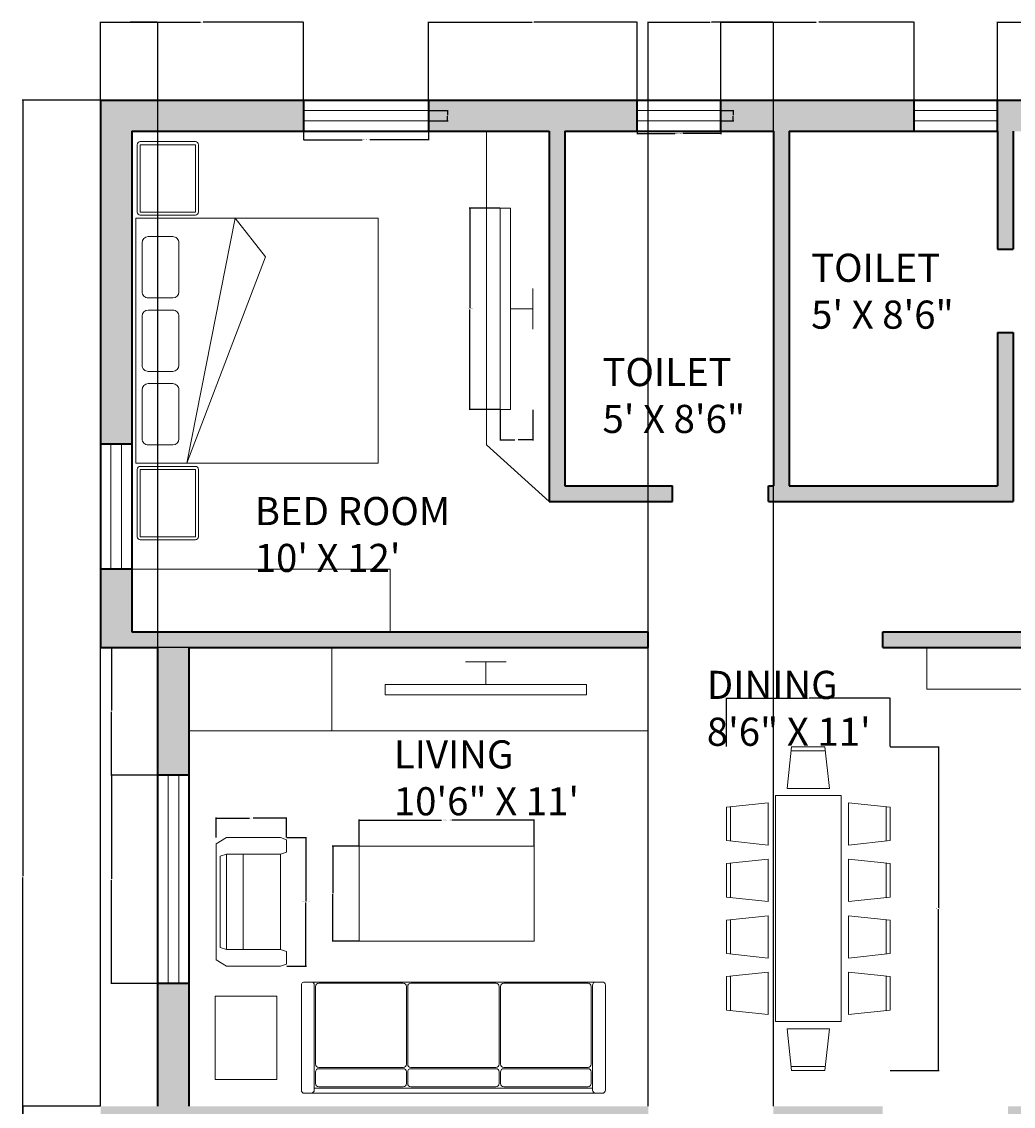
# Model space of a CAD drawing. Units: inches. Extents: x 2 to 2806, y 1095 to 1587.
# Tile 3 of 4: x 2363 to 2648, y 1275 to 1587. Entities that reach past the tile are written whole.
import ezdxf

# ---------------------------------------------------------------- set-up
doc = ezdxf.new("R2010")
doc.units = ezdxf.units.IN
for name, color, linetype, lineweight in [('A-ANNO-DIMS', 2, 'Continuous', 18), ('A-AREA-IDEN', 7, 'Continuous', 25), ('A-EQPM', 8, 'Continuous', 18), ('A-FLOR-CASE', 34, 'Continuous', 18), ('A-FURN', 8, 'Continuous', 18), ('A-GLAZ', 4, 'Continuous', 18), ('A-WALL', 7, 'Continuous', 35)]:
    doc.layers.add(name, color=color, linetype=linetype, lineweight=lineweight)
doc.layers.add('A-WALL-PATT', color=18, linetype='Continuous', lineweight=13, true_color=0x000000)
doc.styles.get("Standard").update_dxf_attribs({"font": 'arial.ttf'})
doc.dimstyles.get("Standard").update_dxf_attribs({"dimtxt": 0.18, "dimasz": 0.18, "dimexe": 0.18, "dimexo": 0.0625, "dimgap": 0.09, "dimtad": 0, "dimtih": 1, "dimtoh": 1, "dimdec": 4, "dimzin": 0, "dimdsep": 46, "dimtxsty": 'Standard', "dimcen": 0.09, "dimadec": 0, "dimazin": 0, "dimtfac": 1, "dimtdec": 4, "dimtofl": 0, "dimtmove": 0, "dimatfit": 3, "dimfxl": 1, "dimtolj": 1, "dimtzin": 0, "dimarcsym": 0})

# ---------------------------------------------------------------- blocks, each defined once
blk = doc.blocks.new('A$C5E814E7E')
for p, q in [((0.593, 1.293), (0.64, 1.736)), ((0.64, 1.736), (0.995, 1.736)), ((0.995, 1.736), (1.043, 1.293)), ((1.193, 1.293), (1.24, 1.736)), ((1.24, 1.736), (1.595, 1.736)), ((1.595, 1.736), (1.643, 1.293)), ((1.793, 1.293), (1.84, 1.736)), ((1.84, 1.736), (2.195, 1.736)), ((2.195, 1.736), (2.243, 1.293)), ((2.393, 1.293), (2.44, 1.736)), ((2.44, 1.736), (2.795, 1.736)), ((2.795, 1.736), (2.843, 1.293)), ((0.636, 1.693), (1, 1.693)), ((1.236, 1.693), (1.6, 1.693)), ((1.836, 1.693), (2.2, 1.693)), ((2.436, 1.693), (2.8, 1.693)), ((1.043, 1.293), (0.593, 1.293)), ((1.643, 1.293), (1.193, 1.293)), ((2.243, 1.293), (1.793, 1.293)), ((2.843, 1.293), (2.393, 1.293)), ((0.518, 1.218), (2.918, 1.218)), ((0.518, 0.518), (0.518, 1.218)), ((2.918, 1.218), (2.918, 0.518)), ((0.443, 1.093), (0, 1.045)), ((0, 1.045), (0, 0.69)), ((0.043, 1.05), (0.043, 0.686)), ((0.443, 0.643), (0.443, 1.093)), ((2.993, 1.093), (3.436, 1.045)), ((2.993, 0.643), (2.993, 1.093)), ((3.393, 1.05), (3.393, 0.686)), ((3.436, 1.045), (3.436, 0.69)), ((0, 0.69), (0.443, 0.643)), ((3.436, 0.69), (2.993, 0.643)), ((2.918, 0.518), (0.518, 0.518)), ((0.593, 0.443), (0.64, 0)), ((1.043, 0.443), (0.593, 0.443)), ((0.995, 0), (1.043, 0.443)), ((1.193, 0.443), (1.24, 0)), ((1.643, 0.443), (1.193, 0.443)), ((1.595, 0), (1.643, 0.443)), ((2.243, 0.443), (1.793, 0.443)), ((1.793, 0.443), (1.84, 0)), ((2.195, 0), (2.243, 0.443)), ((2.393, 0.443), (2.44, 0)), ((2.843, 0.443), (2.393, 0.443)), ((2.795, 0), (2.843, 0.443)), ((0.636, 0.043), (1, 0.043)), ((1.236, 0.043), (1.6, 0.043)), ((1.836, 0.043), (2.2, 0.043)), ((2.436, 0.043), (2.8, 0.043)), ((0.64, 0), (0.995, 0)), ((1.24, 0), (1.595, 0)), ((1.84, 0), (2.195, 0)), ((2.44, 0), (2.795, 0))]:
    blk.add_line(p, q)
blk = doc.blocks.new('A$C0BA509B0')
for p, q in [((0.025, 0.86), (2.325, 0.86)), ((2.25, 0.8385), (2.25, 0.0224)), ((0, 0.025), (0, 0.835)), ((0.1, 0.0219), (0.1, 0.8375)), ((0.1, 0.82), (2.25, 0.82)), ((0.11, 0.695), (0.11, 0.785)), ((0.135, 0.81), (0.7866, 0.81)), ((0.8116, 0.785), (0.8116, 0.695)), ((0.8216, 0.785), (0.8216, 0.695)), ((0.8466, 0.81), (1.5033, 0.81)), ((1.5283, 0.785), (1.5283, 0.695)), ((1.5383, 0.785), (1.5383, 0.695)), ((1.5633, 0.81), (2.215, 0.81)), ((2.24, 0.785), (2.24, 0.695)), ((2.35, 0.835), (2.35, 0.025)), ((0.11, 0.035), (0.11, 0.635)), ((0.135, 0.67), (0.7866, 0.67)), ((0.135, 0.66), (0.7866, 0.66)), ((0.8116, 0.635), (0.8116, 0.035)), ((0.8216, 0.635), (0.8216, 0.035)), ((0.8466, 0.67), (1.5033, 0.67)), ((0.8466, 0.66), (1.5033, 0.66)), ((1.5283, 0.635), (1.5283, 0.035)), ((1.5383, 0.635), (1.5383, 0.035)), ((1.5633, 0.67), (2.215, 0.67)), ((1.5633, 0.66), (2.215, 0.66)), ((2.24, 0.635), (2.24, 0.035)), ((0.7866, 0.01), (0.135, 0.01)), ((1.5033, 0.01), (0.8466, 0.01)), ((2.215, 0.01), (1.5633, 0.01)), ((2.325, 0), (0.025, 0))]:
    blk.add_line(p, q)
for centre, start, end in [((0.025, 0.835), 90, 180), ((0.0751, 0.835), 0, 90), ((2.2752, 0.835), 90, 180), ((2.325, 0.835), 0, 90), ((0.135, 0.785), 90, 180), ((0.7866, 0.785), 0, 90), ((0.8466, 0.785), 90, 180), ((1.5033, 0.785), 0, 90), ((1.5633, 0.785), 90, 180), ((2.215, 0.785), 0, 90), ((0.135, 0.695), 180, 270), ((0.7866, 0.695), 270, 0), ((0.8466, 0.695), 180, 270), ((1.5033, 0.695), 270, 0), ((1.5633, 0.695), 180, 270), ((2.215, 0.695), 270, 0), ((0.135, 0.635), 90, 180), ((0.7866, 0.635), 0, 90), ((0.8466, 0.635), 90, 180), ((1.5033, 0.635), 0, 90), ((1.5633, 0.635), 90, 180), ((2.215, 0.635), 0, 90), ((0.025, 0.025), 180, 270), ((0.0751, 0.025), 270, 0), ((0.135, 0.035), 180, 270), ((0.7866, 0.035), 270, 0), ((0.8466, 0.035), 180, 270), ((1.5033, 0.035), 270, 0), ((1.5633, 0.035), 180, 270), ((2.215, 0.035), 270, 0), ((2.2749, 0.025), 180, 270), ((2.325, 0.025), 270, 0)]:
    blk.add_arc(centre, 0.025, start, end)
blk = doc.blocks.new('A$C61201922')
for p, q in [((0, 0.737), (0.076, 0.864)), ((0.076, 0.864), (1.499, 0.864)), ((0.203, 0.737), (0.229, 0.813)), ((0.229, 0.813), (1.346, 0.813)), ((1.346, 0.813), (1.372, 0.737)), ((1.499, 0.864), (1.575, 0.737)), ((0, 0.076), (0, 0.737)), ((0.203, 0.076), (0.203, 0.737)), ((1.372, 0.737), (0.203, 0.737)), ((1.372, 0.737), (1.372, 0.076)), ((1.575, 0.737), (1.575, 0.076)), ((1.372, 0.533), (0.203, 0.533)), ((0.025, 0), (0, 0.076)), ((0.178, 0), (0.025, 0)), ((0.203, 0.076), (0.178, 0)), ((1.372, 0.076), (0.203, 0.076)), ((1.397, 0), (1.372, 0.076)), ((1.549, 0), (1.397, 0)), ((1.575, 0.076), (1.549, 0))]:
    blk.add_line(p, q)
blk = doc.blocks.new('A$C793B20D3')
for p, q in [((0.625, 0), (0.625, 1.975)), ((2.625, 1.975), (0.625, 1.975)), ((2.625, 0), (2.625, 1.975)), ((2.675, 1.9655), (3.225, 1.9655)), ((0.575, 1.9405), (0.025, 1.9405)), ((0.025, 1.9405), (0.025, 1.4905)), ((0.575, 1.4905), (0.575, 1.9405)), ((0.775, 1.675), (0.775, 1.875)), ((0.825, 1.925), (1.225, 1.925)), ((1.275, 1.675), (1.275, 1.875)), ((1.375, 1.675), (1.375, 1.875)), ((1.425, 1.925), (1.825, 1.925)), ((1.875, 1.675), (1.875, 1.875)), ((1.975, 1.675), (1.975, 1.875)), ((2.025, 1.925), (2.425, 1.925)), ((2.475, 1.675), (2.475, 1.875)), ((2.65, 1.4905), (2.65, 1.9405)), ((3.25, 1.9405), (3.25, 1.4905)), ((0.825, 1.625), (1.225, 1.625)), ((1.425, 1.625), (1.825, 1.625)), ((2.025, 1.625), (2.425, 1.625)), ((0.6256, 1.5604), (2.3107, 0.9169)), ((0.6256, 1.5604), (2.625, 1.1646)), ((0.025, 1.4905), (0.575, 1.4905)), ((3.225, 1.4655), (2.675, 1.4655)), ((2.3107, 0.9169), (2.625, 1.1646)), ((2.625, 0), (0.625, 0))]:
    blk.add_line(p, q)
at = {"flags": 128}
blk.add_lwpolyline([(0, 1.9405), (0, 1.4905, 0.414214), (0.025, 1.4655), (0.575, 1.4655, 0.414214), (0.6, 1.4905), (0.6, 1.9405, 0.414214), (0.575, 1.9655), (0.025, 1.9655, 0.414214)], format="xyb", close=True, dxfattribs=at)
blk.add_lwpolyline([(3.225, 1.9405), (3.225, 1.4905), (2.675, 1.4905), (2.675, 1.9405)], close=True)
for centre, radius, start, end in [((2.675, 1.9405), 0.025, 90, 180), ((3.225, 1.9405), 0.025, 0, 90), ((0.825, 1.875), 0.05, 90, 180), ((1.225, 1.875), 0.05, 0, 90), ((1.425, 1.875), 0.05, 90, 180), ((1.825, 1.875), 0.05, 0, 90), ((2.025, 1.875), 0.05, 90, 180), ((2.425, 1.875), 0.05, 0, 90), ((0.825, 1.675), 0.05, 180, 270), ((1.225, 1.675), 0.05, 270, 0), ((1.425, 1.675), 0.05, 180, 270), ((1.825, 1.675), 0.05, 270, 0), ((2.025, 1.675), 0.05, 180, 270), ((2.425, 1.675), 0.05, 270, 0), ((2.675, 1.4905), 0.025, 180, 270), ((3.225, 1.4905), 0.025, 270, 0)]:
    blk.add_arc(centre, radius, start, end)
blk = doc.blocks.new('WIN-GLAZ-36x9')
for p, q in [((0, 3), (36, 3)), ((0, 0), (36, 0))]:
    blk.add_line(p, q)
blk = doc.blocks.new('WIN-GLAZ-24x9')
for p, q in [((0, 3), (24, 3)), ((0, 0), (24, 0))]:
    blk.add_line(p, q)
blk = doc.blocks.new('TV-FLAT-PANEL')
for p, q in [((23.15, 9.45), (34.81, 9.45)), ((28.98, 3), (28.98, 9.45)), ((0, 3), (57.96, 3)), ((0, 3), (0, 0)), ((0, 0), (57.96, 0)), ((57.96, 0), (57.96, 3))]:
    blk.add_line(p, q)
blk = doc.blocks.new('TABLE-COFFEE-RECT')
blk.add_lwpolyline([(0, 27.27), (50.38, 27.27), (50.38, 0), (0, 0), (0, 27.27)])
blk = doc.blocks.new('*D26')
at = {"layer": 'A-ANNO-DIMS', "color": 0, "lineweight": -2, "transparency": 16777216}
for p, q in [((2444, 1558.15), (2444, 1552.63)), ((2480, 1558.15), (2480, 1552.63)), ((2444.18, 1552.81), (2460.88, 1552.81)), ((2479.82, 1552.81), (2463.12, 1552.81))]:
    blk.add_line(p, q, dxfattribs=at)
at = {"layer": 'A-ANNO-DIMS', "color": 0, "transparency": 16777216}
for points in [[(2444.18, 1552.84), (2444.18, 1552.78), (2444, 1552.81)], [(2479.82, 1552.84), (2479.82, 1552.78), (2480, 1552.81)]]:
    blk.add_solid(points, dxfattribs=at)
at = {"layer": 'Defpoints', "color": 0, "transparency": 16777216}
for p in [(2444, 1558.21), (2480, 1558.21), (2480, 1552.81)]:
    blk.add_point(p, dxfattribs=at)
at = {"layer": 'A-ANNO-DIMS', "color": 0, "transparency": 16777216, "insert": (2462, 1552.81), "char_height": 0.18, "attachment_point": 5}
blk.add_mtext('\\A1;WINDOW 36 TYP.', dxfattribs=at)
blk = doc.blocks.new('*D27')
at = {"layer": 'A-ANNO-DIMS', "color": 0, "lineweight": -2, "transparency": 16777216}
for p, q in [((2480.06, 1561.21), (2485.58, 1561.21)), ((2485.4, 1561.03), (2485.4, 1559.9)), ((2480.06, 1558.21), (2485.58, 1558.21)), ((2485.4, 1558.39), (2485.4, 1559.53))]:
    blk.add_line(p, q, dxfattribs=at)
at = {"layer": 'A-ANNO-DIMS', "color": 0, "transparency": 16777216}
for points in [[(2485.37, 1561.03), (2485.43, 1561.03), (2485.4, 1561.21)], [(2485.37, 1558.39), (2485.43, 1558.39), (2485.4, 1558.21)]]:
    blk.add_solid(points, dxfattribs=at)
at = {"layer": 'Defpoints', "color": 0, "transparency": 16777216}
for p in [(2480, 1561.21), (2485.4, 1561.21), (2480, 1558.21)]:
    blk.add_point(p, dxfattribs=at)
at = {"layer": 'A-ANNO-DIMS', "color": 0, "transparency": 16777216, "insert": (2485.4, 1559.71), "char_height": 0.18, "attachment_point": 5}
blk.add_mtext('\\A1;3 TYP.', dxfattribs=at)
blk = doc.blocks.new('*D28')
at = {"layer": 'A-ANNO-DIMS', "color": 0, "lineweight": -2, "transparency": 16777216}
for p, q in [((2540, 1558.15), (2540, 1554.43)), ((2564, 1558.15), (2564, 1554.43)), ((2540.18, 1554.61), (2550.88, 1554.61)), ((2563.82, 1554.61), (2553.12, 1554.61))]:
    blk.add_line(p, q, dxfattribs=at)
at = {"layer": 'A-ANNO-DIMS', "color": 0, "transparency": 16777216}
for points in [[(2540.18, 1554.64), (2540.18, 1554.58), (2540, 1554.61)], [(2563.82, 1554.64), (2563.82, 1554.58), (2564, 1554.61)]]:
    blk.add_solid(points, dxfattribs=at)
at = {"layer": 'Defpoints', "color": 0, "transparency": 16777216}
for p in [(2540, 1558.21), (2564, 1558.21), (2564, 1554.61)]:
    blk.add_point(p, dxfattribs=at)
at = {"layer": 'A-ANNO-DIMS', "color": 0, "transparency": 16777216, "insert": (2552, 1554.61), "char_height": 0.18, "attachment_point": 5}
blk.add_mtext('\\A1;WINDOW 24 TYP.', dxfattribs=at)
blk = doc.blocks.new('*D29')
at = {"layer": 'A-ANNO-DIMS', "color": 0, "lineweight": -2, "transparency": 16777216}
for p, q in [((2564.06, 1561.21), (2567.78, 1561.21)), ((2567.6, 1561.03), (2567.6, 1559.9)), ((2564.06, 1558.21), (2567.78, 1558.21)), ((2567.6, 1558.39), (2567.6, 1559.53))]:
    blk.add_line(p, q, dxfattribs=at)
at = {"layer": 'A-ANNO-DIMS', "color": 0, "transparency": 16777216}
for points in [[(2567.57, 1561.03), (2567.63, 1561.03), (2567.6, 1561.21)], [(2567.57, 1558.39), (2567.63, 1558.39), (2567.6, 1558.21)]]:
    blk.add_solid(points, dxfattribs=at)
at = {"layer": 'Defpoints', "color": 0, "transparency": 16777216}
for p in [(2564, 1561.21), (2567.6, 1561.21), (2564, 1558.21)]:
    blk.add_point(p, dxfattribs=at)
at = {"layer": 'A-ANNO-DIMS', "color": 0, "transparency": 16777216, "insert": (2567.6, 1559.71), "char_height": 0.18, "attachment_point": 5}
blk.add_mtext('\\A1;3 TYP.', dxfattribs=at)
blk = doc.blocks.new('*D36')
at = {"layer": 'A-ANNO-DIMS', "color": 0, "lineweight": -2, "transparency": 16777216}
for p, q in [((2439.22, 1352.03), (2444.88, 1352.03)), ((2444.7, 1351.85), (2444.7, 1333.72)), ((2444.7, 1315.22), (2444.7, 1333.35)), ((2439.22, 1315.04), (2444.88, 1315.04))]:
    blk.add_line(p, q, dxfattribs=at)
at = {"layer": 'A-ANNO-DIMS', "color": 0, "transparency": 16777216}
for points in [[(2444.67, 1351.85), (2444.73, 1351.85), (2444.7, 1352.03)], [(2444.67, 1315.22), (2444.73, 1315.22), (2444.7, 1315.04)]]:
    blk.add_solid(points, dxfattribs=at)
at = {"layer": 'Defpoints', "color": 0, "transparency": 16777216}
for p in [(2439.15, 1352.03), (2444.7, 1352.03), (2439.15, 1315.04)]:
    blk.add_point(p, dxfattribs=at)
at = {"layer": 'A-ANNO-DIMS', "color": 0, "transparency": 16777216, "insert": (2444.7, 1333.54), "char_height": 0.18, "attachment_point": 5}
blk.add_mtext('\\A1;ARMCHAIR 37 TYP.', dxfattribs=at)
blk = doc.blocks.new('*D37')
at = {"layer": 'A-ANNO-DIMS', "color": 0, "lineweight": -2, "transparency": 16777216}
for p, q in [((2418.87, 1352.09), (2418.87, 1357.76)), ((2419.05, 1357.58), (2428.48, 1357.58)), ((2438.97, 1357.58), (2429.54, 1357.58)), ((2439.15, 1352.09), (2439.15, 1357.76))]:
    blk.add_line(p, q, dxfattribs=at)
at = {"layer": 'A-ANNO-DIMS', "color": 0, "transparency": 16777216}
for points in [[(2419.05, 1357.61), (2419.05, 1357.55), (2418.87, 1357.58)], [(2438.97, 1357.61), (2438.97, 1357.55), (2439.15, 1357.58)]]:
    blk.add_solid(points, dxfattribs=at)
at = {"layer": 'Defpoints', "color": 0, "transparency": 16777216}
for p in [(2418.87, 1357.58), (2418.87, 1352.03), (2439.15, 1352.03)]:
    blk.add_point(p, dxfattribs=at)
at = {"layer": 'A-ANNO-DIMS', "color": 0, "transparency": 16777216, "insert": (2429.01, 1357.58), "char_height": 0.18, "attachment_point": 5}
blk.add_mtext('\\A1;20 TYP.', dxfattribs=at)
blk = doc.blocks.new('*D38')
at = {"layer": 'A-ANNO-DIMS', "color": 0, "lineweight": -2, "transparency": 16777216}
for p, q in [((2500.48, 1533.15), (2491.67, 1533.15)), ((2491.85, 1532.97), (2491.85, 1504.35)), ((2491.85, 1475.37), (2491.85, 1503.99)), ((2500.48, 1475.19), (2491.67, 1475.19))]:
    blk.add_line(p, q, dxfattribs=at)
at = {"layer": 'A-ANNO-DIMS', "color": 0, "transparency": 16777216}
for points in [[(2491.82, 1532.97), (2491.88, 1532.97), (2491.85, 1533.15)], [(2491.82, 1475.37), (2491.88, 1475.37), (2491.85, 1475.19)]]:
    blk.add_solid(points, dxfattribs=at)
at = {"layer": 'Defpoints', "color": 0, "transparency": 16777216}
for p in [(2500.55, 1533.15), (2491.85, 1475.19), (2500.55, 1475.19)]:
    blk.add_point(p, dxfattribs=at)
at = {"layer": 'A-ANNO-DIMS', "color": 0, "transparency": 16777216, "insert": (2491.85, 1504.17), "char_height": 0.18, "attachment_point": 5}
blk.add_mtext('\\A1;TV PANEL 58 TYP.', dxfattribs=at)
blk = doc.blocks.new('*D39')
at = {"layer": 'A-ANNO-DIMS', "color": 0, "lineweight": -2, "transparency": 16777216}
for p, q in [((2500.55, 1475.12), (2500.55, 1466.31)), ((2510, 1475.12), (2510, 1466.31)), ((2500.73, 1466.49), (2504.81, 1466.49)), ((2509.82, 1466.49), (2505.73, 1466.49))]:
    blk.add_line(p, q, dxfattribs=at)
at = {"layer": 'A-ANNO-DIMS', "color": 0, "transparency": 16777216}
for points in [[(2500.73, 1466.52), (2500.73, 1466.46), (2500.55, 1466.49)], [(2509.82, 1466.52), (2509.82, 1466.46), (2510, 1466.49)]]:
    blk.add_solid(points, dxfattribs=at)
at = {"layer": 'Defpoints', "color": 0, "transparency": 16777216}
for p in [(2500.55, 1475.19), (2510, 1475.19), (2510, 1466.49)]:
    blk.add_point(p, dxfattribs=at)
at = {"layer": 'A-ANNO-DIMS', "color": 0, "transparency": 16777216, "insert": (2505.27, 1466.49), "char_height": 0.18, "attachment_point": 5}
blk.add_mtext('\\A1;9 TYP.', dxfattribs=at)
blk = doc.blocks.new('*D40')
at = {"layer": 'A-ANNO-DIMS', "color": 0, "lineweight": -2, "transparency": 16777216}
for p, q in [((2460.01, 1349.59), (2460.01, 1357.26)), ((2460.19, 1357.08), (2483.7, 1357.08)), ((2510.21, 1357.08), (2486.71, 1357.08)), ((2510.39, 1349.59), (2510.39, 1357.26))]:
    blk.add_line(p, q, dxfattribs=at)
at = {"layer": 'A-ANNO-DIMS', "color": 0, "transparency": 16777216}
for points in [[(2460.19, 1357.11), (2460.19, 1357.05), (2460.01, 1357.08)], [(2510.21, 1357.11), (2510.21, 1357.05), (2510.39, 1357.08)]]:
    blk.add_solid(points, dxfattribs=at)
at = {"layer": 'Defpoints', "color": 0, "transparency": 16777216}
for p in [(2510.39, 1357.08), (2460.01, 1349.53), (2510.39, 1349.53)]:
    blk.add_point(p, dxfattribs=at)
at = {"layer": 'A-ANNO-DIMS', "color": 0, "transparency": 16777216, "insert": (2485.2, 1357.08), "char_height": 0.18, "attachment_point": 5}
blk.add_mtext('\\A1;COFFEE TABLE 50 TYP.', dxfattribs=at)
blk = doc.blocks.new('*D41')
at = {"layer": 'A-ANNO-DIMS', "color": 0, "lineweight": -2, "transparency": 16777216}
for p, q in [((2459.95, 1349.53), (2452.27, 1349.53)), ((2452.45, 1349.35), (2452.45, 1336.07)), ((2452.45, 1322.44), (2452.45, 1335.71)), ((2459.95, 1322.26), (2452.27, 1322.26))]:
    blk.add_line(p, q, dxfattribs=at)
at = {"layer": 'A-ANNO-DIMS', "color": 0, "transparency": 16777216}
for points in [[(2452.42, 1349.35), (2452.48, 1349.35), (2452.45, 1349.53)], [(2452.42, 1322.44), (2452.48, 1322.44), (2452.45, 1322.26)]]:
    blk.add_solid(points, dxfattribs=at)
at = {"layer": 'Defpoints', "color": 0, "transparency": 16777216}
for p in [(2452.45, 1349.53), (2460.01, 1349.53), (2460.01, 1322.26)]:
    blk.add_point(p, dxfattribs=at)
at = {"layer": 'A-ANNO-DIMS', "color": 0, "transparency": 16777216, "insert": (2452.45, 1335.89), "char_height": 0.18, "attachment_point": 5}
blk.add_mtext('\\A1;27 TYP.', dxfattribs=at)
blk = doc.blocks.new('*D52')
at = {"layer": 'A-ANNO-DIMS', "color": 0, "lineweight": -2, "transparency": 16777216}
for p, q in [((2612.77, 1378.13), (2626.85, 1378.13)), ((2626.67, 1377.95), (2626.67, 1331.77)), ((2626.67, 1285.22), (2626.67, 1331.4)), ((2612.77, 1285.04), (2626.85, 1285.04))]:
    blk.add_line(p, q, dxfattribs=at)
at = {"layer": 'A-ANNO-DIMS', "color": 0, "transparency": 16777216}
for points in [[(2626.64, 1377.95), (2626.7, 1377.95), (2626.67, 1378.13)], [(2626.64, 1285.22), (2626.7, 1285.22), (2626.67, 1285.04)]]:
    blk.add_solid(points, dxfattribs=at)
at = {"layer": 'Defpoints', "color": 0, "transparency": 16777216}
for p in [(2612.7, 1378.13), (2612.7, 1285.04), (2626.67, 1285.04)]:
    blk.add_point(p, dxfattribs=at)
at = {"layer": 'A-ANNO-DIMS', "color": 0, "transparency": 16777216, "insert": (2626.67, 1331.59), "char_height": 0.18, "attachment_point": 5}
blk.add_mtext('\\A1;DINING SET 93', dxfattribs=at)
blk = doc.blocks.new('*D53')
at = {"layer": 'A-ANNO-DIMS', "color": 0, "lineweight": -2, "transparency": 16777216}
for p, q in [((2565.68, 1378.19), (2565.68, 1392.27)), ((2565.86, 1392.09), (2588.97, 1392.09)), ((2612.52, 1392.09), (2589.41, 1392.09)), ((2612.7, 1378.19), (2612.7, 1392.27))]:
    blk.add_line(p, q, dxfattribs=at)
at = {"layer": 'A-ANNO-DIMS', "color": 0, "transparency": 16777216}
for points in [[(2565.86, 1392.12), (2565.86, 1392.06), (2565.68, 1392.09)], [(2612.52, 1392.12), (2612.52, 1392.06), (2612.7, 1392.09)]]:
    blk.add_solid(points, dxfattribs=at)
at = {"layer": 'Defpoints', "color": 0, "transparency": 16777216}
for p in [(2612.7, 1392.09), (2565.68, 1378.13), (2612.7, 1378.13)]:
    blk.add_point(p, dxfattribs=at)
at = {"layer": 'A-ANNO-DIMS', "color": 0, "transparency": 16777216, "insert": (2589.19, 1392.09), "char_height": 0.18, "attachment_point": 5}
blk.add_mtext('\\A1;47', dxfattribs=at)
blk = doc.blocks.new('*D55')
at = {"layer": 'A-ANNO-DIMS', "color": 0, "lineweight": -2, "transparency": 16777216}
for p, q in [((2411.08, 1370), (2388.6, 1370)), ((2388.78, 1369.82), (2388.78, 1340.18)), ((2388.78, 1310.18), (2388.78, 1339.82)), ((2411.08, 1310), (2388.6, 1310))]:
    blk.add_line(p, q, dxfattribs=at)
at = {"layer": 'A-ANNO-DIMS', "color": 0, "transparency": 16777216}
for points in [[(2388.75, 1369.82), (2388.81, 1369.82), (2388.78, 1370)], [(2388.75, 1310.18), (2388.81, 1310.18), (2388.78, 1310)]]:
    blk.add_solid(points, dxfattribs=at)
at = {"layer": 'Defpoints', "color": 0, "transparency": 16777216}
for p in [(2388.78, 1370), (2411.14, 1370), (2411.14, 1310)]:
    blk.add_point(p, dxfattribs=at)
at = {"layer": 'A-ANNO-DIMS', "color": 0, "transparency": 16777216, "insert": (2388.78, 1340), "char_height": 0.18, "attachment_point": 5}
blk.add_mtext('\\A1;60', dxfattribs=at)
blk = doc.blocks.new('*D56')
at = {"layer": 'A-ANNO-DIMS', "color": 0, "lineweight": -2, "transparency": 16777216}
for p, q in [((2411.08, 1406.71), (2388.6, 1406.71)), ((2388.78, 1406.53), (2388.78, 1388.54)), ((2388.78, 1370.18), (2388.78, 1388.17)), ((2411.08, 1370), (2388.6, 1370))]:
    blk.add_line(p, q, dxfattribs=at)
at = {"layer": 'A-ANNO-DIMS', "color": 0, "transparency": 16777216}
for points in [[(2388.75, 1406.53), (2388.81, 1406.53), (2388.78, 1406.71)], [(2388.75, 1370.18), (2388.81, 1370.18), (2388.78, 1370)]]:
    blk.add_solid(points, dxfattribs=at)
at = {"layer": 'Defpoints', "color": 0, "transparency": 16777216}
for p in [(2388.78, 1406.71), (2411.14, 1406.71), (2411.14, 1370)]:
    blk.add_point(p, dxfattribs=at)
at = {"layer": 'A-ANNO-DIMS', "color": 0, "transparency": 16777216, "insert": (2388.78, 1388.36), "char_height": 0.18, "attachment_point": 5}
blk.add_mtext('\\A1;36.71', dxfattribs=at)
blk = doc.blocks.new('*D57')
at = {"layer": 'A-ANNO-DIMS', "color": 0, "lineweight": -2, "transparency": 16777216}
for p, q in [((2385.580192, 1564.213452), (2363.102692, 1564.213452)), ((2363.282692, 1564.033452), (2363.282692, 1340.893452)), ((2363.282692, 1117.393452), (2363.282692, 1340.533452)), ((2385.580192, 1117.213452), (2363.102692, 1117.213452))]:
    blk.add_line(p, q, dxfattribs=at)
at = {"layer": 'A-ANNO-DIMS', "color": 0, "transparency": 16777216}
for points in [[(2363.252692, 1564.033452), (2363.312692, 1564.033452), (2363.282692, 1564.213452)], [(2363.252692, 1117.393452), (2363.312692, 1117.393452), (2363.282692, 1117.213452)]]:
    blk.add_solid(points, dxfattribs=at)
at = {"layer": 'Defpoints', "color": 0, "transparency": 16777216}
for p in [(2363.282692, 1564.213452), (2385.642692, 1564.213452), (2385.642692, 1117.213452)]:
    blk.add_point(p, dxfattribs=at)
at = {"layer": 'A-ANNO-DIMS', "color": 0, "transparency": 16777216, "insert": (2363.282692, 1340.713452), "char_height": 0.18, "attachment_point": 5}
blk.add_mtext('\\A1;447', dxfattribs=at)
blk = doc.blocks.new('*D62')
at = {"layer": 'A-ANNO-DIMS', "color": 0, "lineweight": -2, "transparency": 16777216}
for p, q in [((2385.64, 1564.28), (2385.64, 1586.75)), ((2385.82, 1586.57), (2414.43, 1586.57)), ((2443.82, 1586.57), (2415.21, 1586.57)), ((2444, 1564.28), (2444, 1586.75))]:
    blk.add_line(p, q, dxfattribs=at)
at = {"layer": 'A-ANNO-DIMS', "color": 0, "transparency": 16777216}
for points in [[(2385.82, 1586.6), (2385.82, 1586.54), (2385.64, 1586.57)], [(2443.82, 1586.6), (2443.82, 1586.54), (2444, 1586.57)]]:
    blk.add_solid(points, dxfattribs=at)
at = {"layer": 'Defpoints', "color": 0, "transparency": 16777216}
for p in [(2444, 1586.57), (2385.64, 1564.21), (2444, 1564.21)]:
    blk.add_point(p, dxfattribs=at)
at = {"layer": 'A-ANNO-DIMS', "color": 0, "transparency": 16777216, "insert": (2414.82, 1586.57), "char_height": 0.18, "attachment_point": 5}
blk.add_mtext('\\A1;58.36', dxfattribs=at)
blk = doc.blocks.new('*D63')
at = {"layer": 'A-ANNO-DIMS', "color": 0, "lineweight": -2, "transparency": 16777216}
for p, q in [((2480, 1564.28), (2480, 1586.75)), ((2480.18, 1586.57), (2509.78, 1586.57)), ((2539.82, 1586.57), (2510.22, 1586.57)), ((2540, 1564.28), (2540, 1586.75))]:
    blk.add_line(p, q, dxfattribs=at)
at = {"layer": 'A-ANNO-DIMS', "color": 0, "transparency": 16777216}
for points in [[(2480.18, 1586.6), (2480.18, 1586.54), (2480, 1586.57)], [(2539.82, 1586.6), (2539.82, 1586.54), (2540, 1586.57)]]:
    blk.add_solid(points, dxfattribs=at)
at = {"layer": 'Defpoints', "color": 0, "transparency": 16777216}
for p in [(2540, 1586.57), (2480, 1564.21), (2540, 1564.21)]:
    blk.add_point(p, dxfattribs=at)
at = {"layer": 'A-ANNO-DIMS', "color": 0, "transparency": 16777216, "insert": (2510, 1586.57), "char_height": 0.18, "attachment_point": 5}
blk.add_mtext('\\A1;60', dxfattribs=at)
blk = doc.blocks.new('*D64')
at = {"layer": 'A-ANNO-DIMS', "color": 0, "lineweight": -2, "transparency": 16777216}
for p, q in [((2564, 1564.28), (2564, 1586.75)), ((2564.18, 1586.57), (2591.43, 1586.57)), ((2619.46, 1586.57), (2592.21, 1586.57)), ((2619.64, 1564.28), (2619.64, 1586.75))]:
    blk.add_line(p, q, dxfattribs=at)
at = {"layer": 'A-ANNO-DIMS', "color": 0, "transparency": 16777216}
for points in [[(2564.18, 1586.6), (2564.18, 1586.54), (2564, 1586.57)], [(2619.46, 1586.6), (2619.46, 1586.54), (2619.64, 1586.57)]]:
    blk.add_solid(points, dxfattribs=at)
at = {"layer": 'Defpoints', "color": 0, "transparency": 16777216}
for p in [(2619.64, 1586.57), (2564, 1564.21), (2619.64, 1564.21)]:
    blk.add_point(p, dxfattribs=at)
at = {"layer": 'A-ANNO-DIMS', "color": 0, "transparency": 16777216, "insert": (2591.82, 1586.57), "char_height": 0.18, "attachment_point": 5}
blk.add_mtext('\\A1;55.64', dxfattribs=at)
blk = doc.blocks.new('*D65')
at = {"layer": 'A-ANNO-DIMS', "color": 0, "lineweight": -2, "transparency": 16777216}
for p, q in [((2643.64, 1564.28), (2643.64, 1586.75)), ((2643.82, 1586.57), (2650.37, 1586.57)), ((2657.82, 1586.57), (2651.28, 1586.57)), ((2658, 1564.28), (2658, 1586.75))]:
    blk.add_line(p, q, dxfattribs=at)
at = {"layer": 'A-ANNO-DIMS', "color": 0, "transparency": 16777216}
for points in [[(2643.82, 1586.6), (2643.82, 1586.54), (2643.64, 1586.57)], [(2657.82, 1586.6), (2657.82, 1586.54), (2658, 1586.57)]]:
    blk.add_solid(points, dxfattribs=at)
at = {"layer": 'Defpoints', "color": 0, "transparency": 16777216}
for p in [(2658, 1586.57), (2643.64, 1564.21), (2658, 1564.21)]:
    blk.add_point(p, dxfattribs=at)
at = {"layer": 'A-ANNO-DIMS', "color": 0, "transparency": 16777216, "insert": (2650.82, 1586.57), "char_height": 0.18, "attachment_point": 5}
blk.add_mtext('\\A1;14.357', dxfattribs=at)
blk = doc.blocks.new('*D70')
at = {"layer": 'A-ANNO-DIMS', "color": 0, "lineweight": -2, "transparency": 16777216}
for p, q in [((2385.64, 1274.78), (2385.64, 1586.75)), ((2385.82, 1586.57), (2393.58, 1586.57)), ((2401.96, 1586.57), (2394.21, 1586.57)), ((2402.14, 1274.78), (2402.14, 1586.75))]:
    blk.add_line(p, q, dxfattribs=at)
at = {"layer": 'A-ANNO-DIMS', "color": 0, "transparency": 16777216}
for points in [[(2385.82, 1586.6), (2385.82, 1586.54), (2385.64, 1586.57)], [(2401.96, 1586.6), (2401.96, 1586.54), (2402.14, 1586.57)]]:
    blk.add_solid(points, dxfattribs=at)
at = {"layer": 'Defpoints', "color": 0, "transparency": 16777216}
for p in [(2402.14, 1586.57), (2385.64, 1274.71), (2402.14, 1274.71)]:
    blk.add_point(p, dxfattribs=at)
at = {"layer": 'A-ANNO-DIMS', "color": 0, "transparency": 16777216, "insert": (2393.89, 1586.57), "char_height": 0.18, "attachment_point": 5}
blk.add_mtext('\\A1;16.5', dxfattribs=at)
blk = doc.blocks.new('*D71')
at = {"layer": 'A-ANNO-DIMS', "color": 0, "lineweight": -2, "transparency": 16777216}
for p, q in [((2543.14, 1274.78), (2543.14, 1586.75)), ((2543.32, 1586.57), (2560.92, 1586.57)), ((2578.96, 1586.57), (2561.36, 1586.57)), ((2579.14, 1274.78), (2579.14, 1586.75))]:
    blk.add_line(p, q, dxfattribs=at)
at = {"layer": 'A-ANNO-DIMS', "color": 0, "transparency": 16777216}
for points in [[(2543.32, 1586.6), (2543.32, 1586.54), (2543.14, 1586.57)], [(2578.96, 1586.6), (2578.96, 1586.54), (2579.14, 1586.57)]]:
    blk.add_solid(points, dxfattribs=at)
at = {"layer": 'Defpoints', "color": 0, "transparency": 16777216}
for p in [(2579.14, 1586.57), (2543.14, 1274.71), (2579.14, 1274.71)]:
    blk.add_point(p, dxfattribs=at)
at = {"layer": 'A-ANNO-DIMS', "color": 0, "transparency": 16777216, "insert": (2561.14, 1586.57), "char_height": 0.18, "attachment_point": 5}
blk.add_mtext('\\A1;36', dxfattribs=at)
blk = doc.blocks.new('*D72')
at = {"layer": 'A-ANNO-DIMS', "color": 0, "lineweight": -2, "transparency": 16777216}
for p, q in [((2385.58, 1274.71), (2363.1, 1274.71)), ((2363.28, 1274.53), (2363.28, 1196.15)), ((2363.28, 1117.39), (2363.28, 1195.78)), ((2385.58, 1117.21), (2363.1, 1117.21))]:
    blk.add_line(p, q, dxfattribs=at)
at = {"layer": 'A-ANNO-DIMS', "color": 0, "transparency": 16777216}
for points in [[(2363.25, 1274.53), (2363.31, 1274.53), (2363.28, 1274.71)], [(2363.25, 1117.39), (2363.31, 1117.39), (2363.28, 1117.21)]]:
    blk.add_solid(points, dxfattribs=at)
at = {"layer": 'Defpoints', "color": 0, "transparency": 16777216}
for p in [(2363.28, 1274.71), (2385.64, 1274.71), (2385.64, 1117.21)]:
    blk.add_point(p, dxfattribs=at)
at = {"layer": 'A-ANNO-DIMS', "color": 0, "transparency": 16777216, "insert": (2363.28, 1195.96), "char_height": 0.18, "attachment_point": 5}
blk.add_mtext('\\A1;157.5', dxfattribs=at)

msp = doc.modelspace()

# ---------------------------------------------------------------- hatches: boundary and pattern name
at = {"layer": 'A-WALL-PATT'}
h = msp.add_hatch(color=256, dxfattribs=at)
h.dxf.hatch_style = 1
h.paths.add_polyline_path([(2444, 1564.2135), (2385.6427, 1564.2135), (2385.6427, 1465.2135), (2394.6427, 1465.2135), (2394.6427, 1555.2135), (2444, 1555.2135)])
h.paths.add_polyline_path([(2540, 1564.2135), (2480, 1564.2135), (2480, 1555.2135), (2514.6427, 1555.2135), (2514.6427, 1448.7135), (2550.1001, 1448.7135), (2550.1001, 1453.2135), (2519.1427, 1453.2135), (2519.1427, 1555.2135), (2540, 1555.2135)])
h.paths.add_polyline_path([(2619.6427, 1564.2135), (2564, 1564.2135), (2564, 1555.2135), (2579.1427, 1555.2135), (2579.1427, 1453.2135), (2577.7846, 1453.2135), (2577.7846, 1448.7135), (2648.1427, 1448.7135), (2648.1427, 1497.3535), (2643.6427, 1497.3535), (2643.6427, 1453.2135), (2583.6427, 1453.2135), (2583.6427, 1555.2135), (2619.6427, 1555.2135)])
h.paths.add_polyline_path([(2658, 1564.2135), (2643.6427, 1564.2135), (2643.6427, 1555.2135), (2643.6427, 1521.3535), (2648.1427, 1521.3535), (2648.1427, 1555.2135), (2658, 1555.2135)])
h.paths.add_polyline_path([(2783.1427, 1564.2135), (2730, 1564.2135), (2730, 1555.2135), (2774.1427, 1555.2135), (2774.1427, 1465.3633), (2783.1427, 1465.3633)])
h.paths.add_polyline_path([(2783.1427, 1429.3633), (2774.1427, 1429.3633), (2774.1427, 1411.2135), (2610.5887, 1411.2135), (2610.5887, 1406.7135), (2774.1427, 1406.7135), (2774.1427, 1394.7135), (2783.1427, 1394.7135)])
h.paths.add_polyline_path([(2783.1427, 1358.7135), (2774.1427, 1358.7135), (2774.1427, 1336), (2783.1427, 1336)])
h.paths.add_polyline_path([(2783.1427, 1300), (2774.1427, 1300), (2774.1427, 1274.7135), (2646.5887, 1274.7135), (2646.5887, 1270.2135), (2774.1427, 1270.2135), (2774.1427, 1126.2135), (2750.1427, 1126.2135), (2750.1427, 1117.2135), (2783.1427, 1117.2135)])
h.paths.add_polyline_path([(2607.6427, 1126.2135), (2567.1427, 1126.2135), (2567.1427, 1117.2135), (2607.6427, 1117.2135)])
h.paths.add_polyline_path([(2714.1427, 1126.2135), (2643.6427, 1126.2135), (2643.6427, 1117.2135), (2714.1427, 1117.2135)])
h.paths.add_polyline_path([(2607.6427, 1270.2135), (2610.5887, 1270.2135), (2610.5887, 1274.7135), (2579.1427, 1274.7135), (2579.1427, 1270.2135), (2603.1427, 1270.2135), (2603.1427, 1232.7135), (2538.6427, 1232.7135), (2538.6427, 1126.2135), (2543.1427, 1126.2135), (2543.1427, 1228.2135), (2603.1427, 1228.2135), (2603.1427, 1189.2001), (2607.6427, 1189.2001)])
h.paths.add_polyline_path([(2543.1427, 1126.2135), (2514.6427, 1126.2135), (2514.6427, 1117.2135), (2543.1427, 1117.2135)], flags=17)
h.paths.add_polyline_path([(2418.6427, 1126.2135), (2394.6427, 1126.2135), (2394.6427, 1270.2135), (2418.6427, 1270.2135), (2543.1427, 1270.2135), (2543.1427, 1274.7135), (2411.1427, 1274.7135), (2411.1427, 1310), (2402.1427, 1310), (2402.1427, 1274.7135), (2385.6427, 1274.7135), (2385.6427, 1117.2135), (2418.6427, 1117.2135)])
h.paths.add_polyline_path([(2543.1427, 1411.2135), (2394.6427, 1411.2135), (2394.6427, 1429.2135), (2385.6427, 1429.2135), (2385.6427, 1406.7135), (2402.1427, 1406.7135), (2402.1427, 1370), (2411.1427, 1370), (2411.1427, 1406.7135), (2543.1427, 1406.7135)])

# ---------------------------------------------------------------- linework, layer by layer
at = {"layer": 'A-FLOR-CASE'}
for p, q in [((2496.6427, 1555.2135), (2496.6427, 1464.9696)), ((2514.6427, 1448.7135), (2496.6427, 1464.9696)), ((2468.8927, 1429.2135), (2394.6427, 1429.2135)), ((2468.8927, 1411.2135), (2468.8927, 1429.2135)), ((2452.1427, 1382.7135), (2452.1427, 1406.7135)), ((2543.1427, 1406.7135), (2543.1427, 1382.7135)), ((2623.3219, 1394.7135), (2623.3219, 1406.7135)), ((2783.1427, 1394.7135), (2623.3219, 1394.7135)), ((2543.1427, 1382.7135), (2411.1427, 1382.7135))]:
    msp.add_line(p, q, dxfattribs=at)
at = {"layer": 'A-FURN'}
for p, q in [((2418.6515, 1306.4228), (2436.3514, 1306.4228)), ((2418.6515, 1282.3818), (2418.6515, 1306.4228)), ((2436.3514, 1306.4228), (2436.3514, 1282.3818)), ((2436.3514, 1282.3818), (2418.6515, 1282.3818))]:
    msp.add_line(p, q, dxfattribs=at)
at = {"layer": 'A-GLAZ'}
for p, q in [((2405.1427, 1310), (2405.1427, 1370)), ((2408.1427, 1310), (2408.1427, 1370))]:
    msp.add_line(p, q, dxfattribs=at)
at = {"layer": 'A-WALL'}
for p, q in [((2385.6427, 1564.2135), (2783.1427, 1564.2135)), ((2385.6427, 1564.2135), (2385.6427, 1406.7135)), ((2444, 1564.2135), (2444, 1555.2135)), ((2480, 1564.2135), (2480, 1555.2135)), ((2540, 1555.2135), (2540, 1564.2135)), ((2564, 1555.2135), (2564, 1564.2135)), ((2619.6427, 1555.2135), (2619.6427, 1564.2135)), ((2643.6427, 1555.2135), (2643.6427, 1564.2135)), ((2394.6427, 1555.2135), (2394.6427, 1411.2135)), ((2394.6427, 1555.2135), (2514.6427, 1555.2135)), ((2514.6427, 1555.2135), (2514.6427, 1448.7135)), ((2519.1427, 1555.2135), (2519.1427, 1453.2135)), ((2519.1427, 1555.2135), (2579.1427, 1555.2135)), ((2579.1427, 1555.2135), (2579.1427, 1453.2135)), ((2583.6427, 1555.2135), (2583.6427, 1453.2135)), ((2583.6427, 1555.2135), (2643.6427, 1555.2135)), ((2643.6427, 1555.2135), (2643.6427, 1521.3535)), ((2648.1427, 1555.2135), (2648.1427, 1521.3535)), ((2643.6427, 1521.3535), (2648.1427, 1521.3535)), ((2643.6427, 1497.3535), (2648.1427, 1497.3535)), ((2643.6427, 1497.3535), (2643.6427, 1453.2135)), ((2648.1427, 1497.3535), (2648.1427, 1448.7135)), ((2394.6427, 1465.2135), (2385.6427, 1465.2135)), ((2519.1427, 1453.2135), (2550.1001, 1453.2135)), ((2550.1001, 1448.7135), (2550.1001, 1453.2135)), ((2577.7846, 1448.7135), (2577.7846, 1453.2135)), ((2577.7846, 1453.2135), (2579.1427, 1453.2135)), ((2583.6427, 1453.2135), (2643.6427, 1453.2135)), ((2514.6427, 1448.7135), (2550.1001, 1448.7135)), ((2577.7846, 1448.7135), (2648.1427, 1448.7135)), ((2394.6427, 1429.2135), (2385.6427, 1429.2135)), ((2394.6427, 1411.2135), (2543.1427, 1411.2135)), ((2543.1427, 1406.7135), (2543.1427, 1411.2135)), ((2610.5887, 1406.7135), (2610.5887, 1411.2135)), ((2610.5887, 1411.2135), (2774.1427, 1411.2135)), ((2385.6427, 1406.7135), (2402.1427, 1406.7135)), ((2402.1427, 1274.7135), (2402.1427, 1406.7135)), ((2411.1427, 1274.7135), (2411.1427, 1406.7135)), ((2411.1427, 1406.7135), (2543.1427, 1406.7135)), ((2610.5887, 1406.7135), (2774.1427, 1406.7135)), ((2411.1427, 1370), (2402.1427, 1370)), ((2411.1427, 1310), (2402.1427, 1310))]:
    msp.add_line(p, q, dxfattribs=at)

# ---------------------------------------------------------------- block references
at = {"layer": 'A-EQPM', "rotation": 270.0000000000005}
msp.add_blockref('TV-FLAT-PANEL', (2500.5452, 1533.1486), dxfattribs=at)
at = {"layer": 'A-EQPM'}
msp.add_blockref('TV-FLAT-PANEL', (2467.4903, 1393.1), dxfattribs=at)
at = {"layer": 'A-FURN'}
for name, p, xscale, yscale, zscale, rotation in [('A$C793B20D3', (2465.4562, 1437.6755), 35.25, 35.25, 35.25, 89.99999999999999), ('A$C5E814E7E', (2565.6755, 1378.1307), 27.09440126805379, 27.09440126805379, 27.09440126805379, 270), ('A$C61201922', (2439.1536, 1315.0433), 23.48594063424203, 23.48594063424203, 23.48594063424203, 90), ('A$C0BA509B0', (2530.859, 1310.4747), 37.21767998259284, 37.21767998259284, 37.21767998259284, 180)]:
    msp.add_blockref(name, p, dxfattribs=dict(at, xscale=xscale, yscale=yscale, zscale=zscale, rotation=rotation))
msp.add_blockref('TABLE-COFFEE-RECT', (2460.0116, 1322.2607), dxfattribs=at)
at = {"layer": 'A-GLAZ'}
for name, p in [('WIN-GLAZ-36x9', (2444, 1558.2135)), ('WIN-GLAZ-24x9', (2540, 1558.2135)), ('WIN-GLAZ-24x9', (2619.6427, 1558.2135))]:
    msp.add_blockref(name, p, dxfattribs=at)
at = {"layer": 'A-GLAZ', "rotation": 90.00000000000134}
msp.add_blockref('WIN-GLAZ-36x9', (2391.6427, 1429.2135), dxfattribs=at)

# ---------------------------------------------------------------- texts
at = {"layer": 'A-AREA-IDEN', "char_height": 8.08939, "attachment_point": 1}
for s, insert in [('TOILET\\P5\' X 8\'6"', (2590, 1520)), ('TOILET\\P5\' X 8\'6"', (2530, 1490)), ("BED ROOM \\P10' X 12'", (2430, 1450)), ('DINING\\P8\'6" X 11\'', (2560, 1400))]:
    msp.add_mtext(s, dxfattribs=dict(at, insert=insert))
at = {"layer": 'A-AREA-IDEN', "insert": (2470, 1380), "char_height": 8.089392, "width": 73.417451, "attachment_point": 1}
msp.add_mtext('LIVING\\P10\'6" X 11\'', dxfattribs=at)

# ---------------------------------------------------------------- dimensions: what is measured, and where the dimension line sits
at = {"layer": 'A-ANNO-DIMS'}
for base, p1, p2, override, picture, middle in [((2444, 1586.5735), (2385.6427, 1564.2135), (2444, 1564.2135), {"dimdec": 2, "dimlfac": 1, "dimrnd": 0, "dimzin": 0, "dimdsep": 46, "dimlunit": 2}, '*D62', (2414.8213, 1586.5735)), ((2402.1427, 1586.5735), (2385.6427, 1274.7135), (2402.1427, 1274.7135), {"dimdec": 1, "dimlfac": 1, "dimrnd": 0, "dimzin": 0, "dimdsep": 46, "dimlunit": 2}, '*D70', (2393.8927, 1586.5735)), ((2540, 1586.5735), (2480, 1564.2135), (2540, 1564.2135), {"dimdec": 0, "dimlfac": 1, "dimrnd": 0, "dimzin": 0, "dimdsep": 46, "dimlunit": 2}, '*D63', (2510, 1586.5735)), ((2579.1427, 1586.5735), (2543.1427, 1274.7135), (2579.1427, 1274.7135), {"dimdec": 0, "dimlfac": 1, "dimrnd": 0, "dimzin": 0, "dimdsep": 46, "dimlunit": 2}, '*D71', (2561.1427, 1586.5735)), ((2619.6427, 1586.5735), (2564, 1564.2135), (2619.6427, 1564.2135), {"dimdec": 2, "dimlfac": 1, "dimrnd": 0, "dimzin": 0, "dimdsep": 46, "dimlunit": 2}, '*D64', (2591.8213, 1586.5735)), ((2658, 1586.5735), (2643.6427, 1564.2135), (2658, 1564.2135), {"dimdec": 3, "dimlfac": 1, "dimrnd": 0, "dimzin": 0, "dimdsep": 46, "dimlunit": 2}, '*D65', (2650.8213, 1586.5735)), ((2612.705, 1392.0942), (2565.6755, 1378.1307), (2612.705, 1378.1307), {"dimdec": 0, "dimlfac": 1, "dimrnd": 0, "dimzin": 0, "dimdsep": 46, "dimlunit": 2}, '*D53', (2589.1902, 1392.0942))]:
    dim = msp.add_linear_dim(base=base, p1=p1, p2=p2, dimstyle='Standard', override=override, dxfattribs=at)
    dim.commit()
    dim.dimension.update_dxf_attribs({"geometry": picture, "text_midpoint": middle})
for base, p1, p2, override, picture, middle in [((2363.2827, 1564.2135), (2385.6427, 1117.2135), (2385.6427, 1564.2135), {"dimdec": 0, "dimlfac": 1, "dimrnd": 0, "dimzin": 0, "dimdsep": 46, "dimlunit": 2}, '*D57', (2363.2827, 1340.7135)), ((2388.7827, 1406.7135), (2411.1427, 1370), (2411.1427, 1406.7135), {"dimdec": 2, "dimlfac": 1, "dimrnd": 0, "dimzin": 0, "dimdsep": 46, "dimlunit": 2}, '*D56', (2388.7827, 1388.3567)), ((2388.7827, 1370), (2411.1427, 1310), (2411.1427, 1370), {"dimdec": 0, "dimlfac": 1, "dimrnd": 0, "dimzin": 0, "dimdsep": 46, "dimlunit": 2}, '*D55', (2388.7827, 1340)), ((2363.2827, 1274.7135), (2385.6427, 1117.2135), (2385.6427, 1274.7135), {"dimdec": 1, "dimlfac": 1, "dimrnd": 0, "dimzin": 0, "dimdsep": 46, "dimlunit": 2}, '*D72', (2363.2827, 1195.9635))]:
    dim = msp.add_linear_dim(base=base, p1=p1, p2=p2, angle=90, dimstyle='Standard', override=override, dxfattribs=at)
    dim.commit()
    dim.dimension.update_dxf_attribs({"geometry": picture, "text_midpoint": middle})
for base, p1, p2, angle, text, picture, middle in [((2485.4, 1561.2135), (2480, 1558.2135), (2480, 1561.2135), 90, '<> TYP.', '*D27', (2485.4, 1559.7135)), ((2567.6, 1561.2135), (2564, 1558.2135), (2564, 1561.2135), 90, '<> TYP.', '*D29', (2567.6, 1559.7135)), ((2491.851, 1475.1873), (2500.5452, 1533.1486), (2500.5452, 1475.1873), 270, 'TV PANEL <> TYP.', '*D38', (2491.851, 1504.168)), ((2626.6685, 1285.0407), (2612.705, 1378.1307), (2612.705, 1285.0407), 270, 'DINING SET <>', '*D52', (2626.6685, 1331.5857)), ((2418.8712, 1357.5768), (2439.1536, 1352.029), (2418.8712, 1352.029), 180, '<> TYP.', '*D37', (2429.0124, 1357.5768)), ((2444.7015, 1352.029), (2439.1536, 1315.0433), (2439.1536, 1352.029), 90, 'ARMCHAIR <> TYP.', '*D36', (2444.7015, 1333.5361)), ((2452.4549, 1349.5263), (2460.0116, 1322.2607), (2460.0116, 1349.5263), 90, '<> TYP.', '*D41', (2452.4549, 1335.8935))]:
    dim = msp.add_linear_dim(base=base, p1=p1, p2=p2, angle=angle, text=text, dimstyle='Standard', override={"dimdec": 0, "dimlfac": 1, "dimrnd": 0, "dimzin": 0, "dimdsep": 46, "dimlunit": 2}, dxfattribs=at)
    dim.commit()
    dim.dimension.update_dxf_attribs({"geometry": picture, "text_midpoint": middle})
for base, p1, p2, text, picture, middle in [((2480, 1552.8135), (2444, 1558.2135), (2480, 1558.2135), 'WINDOW <> TYP.', '*D26', (2462, 1552.8135)), ((2564, 1554.6135), (2540, 1558.2135), (2564, 1558.2135), 'WINDOW <> TYP.', '*D28', (2552, 1554.6135)), ((2510, 1466.4932), (2500.5452, 1475.1873), (2510, 1475.1873), '<> TYP.', '*D39', (2505.2726, 1466.4932)), ((2510.3897, 1357.0831), (2460.0116, 1349.5263), (2510.3897, 1349.5263), 'COFFEE TABLE <> TYP.', '*D40', (2485.2007, 1357.0831))]:
    dim = msp.add_linear_dim(base=base, p1=p1, p2=p2, text=text, dimstyle='Standard', override={"dimdec": 0, "dimlfac": 1, "dimrnd": 0, "dimzin": 0, "dimdsep": 46, "dimlunit": 2}, dxfattribs=at)
    dim.commit()
    dim.dimension.update_dxf_attribs({"geometry": picture, "text_midpoint": middle})

doc.saveas('drawing.dxf')
